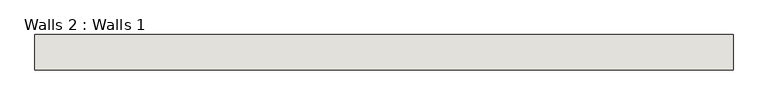
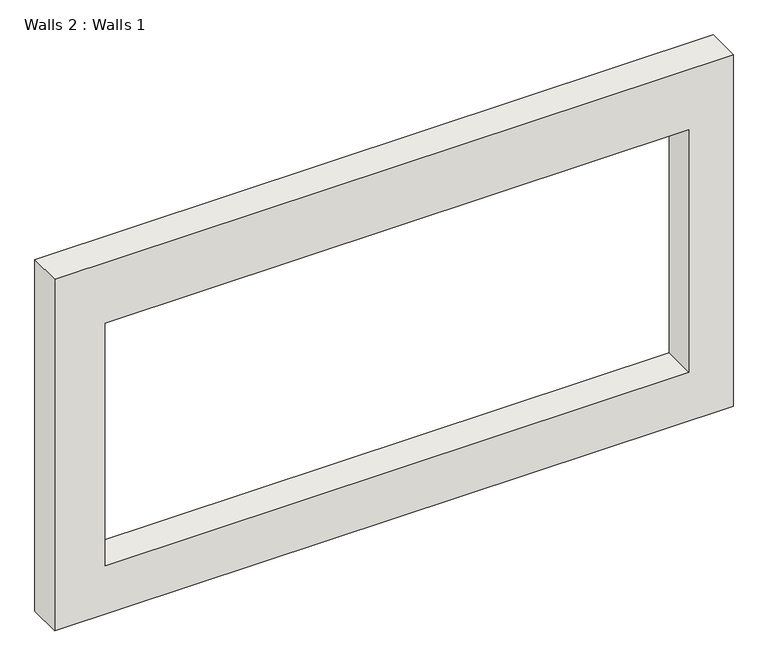
"""IFC4 building model written with IfcOpenShell, lengths in millimetres: wall geometry, Walls 2 : Walls 1."""

from ifc_helpers import new_model, si_unit, frame, origin, place, context, project, spatial, polyline, outline, extrude, source, transform, mapped, element, save


def walls_2_walls_1_38dba3ac(model_context):
    return source(origin(), model_context, "Body", "SweptSolid", [
        extrude(outline(polyline([(16115.6224886, -197.9561565), (16115.6224886, -6243.1561565), (12801.6, -6243.1561565), (12801.6, -197.9561565), (16115.6224886, -197.9561565)]), holes=[polyline([(15544.8, -5793.4328139), (15544.8, -592.6598068), (13258.8733744, -592.6598068), (13258.8733744, -5793.4328139), (15544.8, -5793.4328139)])]), frame((0.0, 1141.3485991, 0.0), z_axis=(0.0, 1.0, 0.0), x_axis=(0.0, 0.0, 1.0)), (0.0, 0.0, 1.0), 304.8),
    ])


if __name__ == "__main__":
    model = new_model("IFC4")
    model_context = context("Model", 3, world=origin())
    ifc_project = project(units=[si_unit("LENGTHUNIT", "METRE", prefix="MILLI")], contexts=[model_context])
    site = spatial("IfcSite", under=ifc_project)
    building = spatial("IfcBuilding", under=site)
    placement = place(None, origin())
    walls_2_walls_1_shape = walls_2_walls_1_38dba3ac(model_context)
    element("IfcWall", 1, ObjectType="Walls 2 : Walls 1", at=placement, inside=building, context=model_context, shape_type="MappedRepresentation", body=[
        mapped(walls_2_walls_1_shape, transform((0.0, 0.0, 0.0), x_axis=(1.0, 0.0, 0.0), y_axis=(0.0, 1.0, 0.0), z_axis=(0.0, 0.0, 1.0))),
    ])
    save(model, "model.ifc")

# Revit data of these elements
# Element 1 (IfcWall, "Walls 2 : Walls 1")
#   Materials on its faces: "Default Wall"
# Materials
#   "Default Wall": colour RGB 128 128 128, transparency 0
